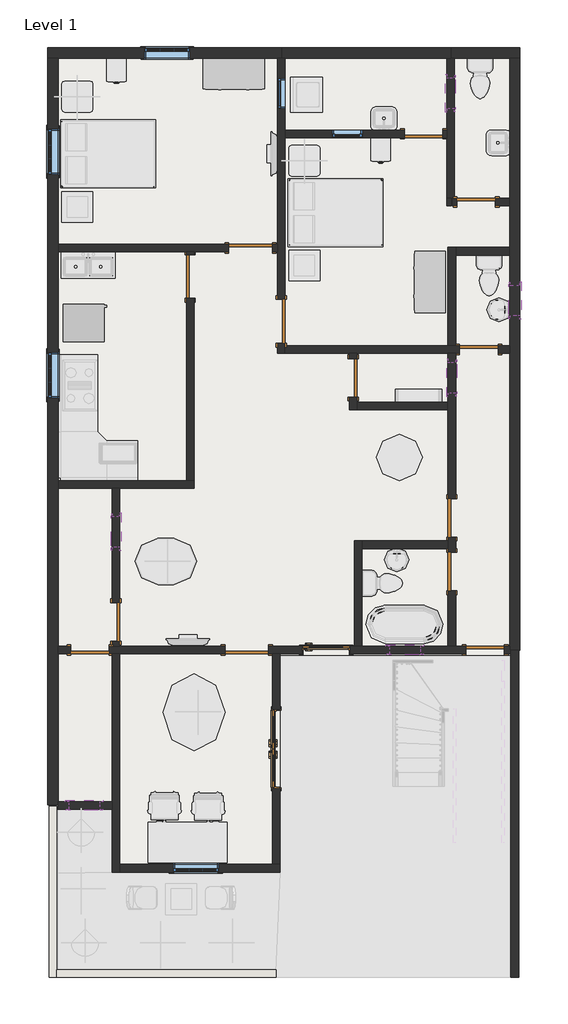
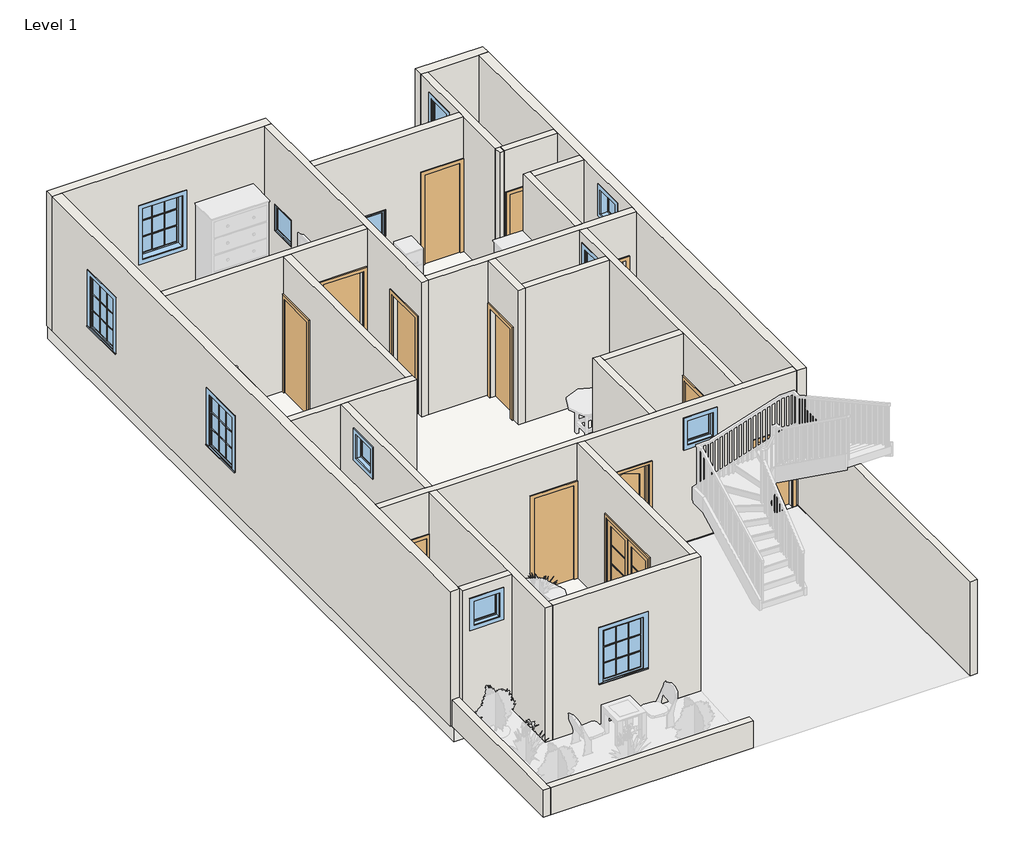
# One storey, part 1 of 3: 30 walls, 15 doors, 12 windows, 1 slab.
"""IFC4 building model written with IfcOpenShell, lengths in millimetres."""

from ifc_helpers import new_model, si_unit, frame, origin, origin_with_axes, place, context, project, spatial, polyline, outline, extrude, faceted_brep, transform, mapped, element, save
from components import door_5d363d20, door_94998e6c, door_1a1933ce, door_255cab33, door_059fdd7e, door_b6e9fca3, door_99d96fc5, window_29c06734, window_5c190c7e, window_aff1bc2a, window_3d781103, window_e41d21a6

model = new_model("IFC4")

# Units and contexts
model_context = context("Model", 3, world=origin())
ifc_project = project(units=[si_unit("LENGTHUNIT", "METRE", prefix="MILLI")], contexts=[model_context])

# Site, building, storey
site = spatial("IfcSite", under=ifc_project)
building = spatial("IfcBuilding", under=site)
storey = spatial("IfcBuildingStorey", under=building, Name="Level 1", Elevation=0.0)

# Doors
placement = place(None, origin())
door_shape = door_5d363d20(model_context)
element("IfcDoor", 1, ObjectType="36\" x 80\"", at=placement, inside=storey, context=model_context, shape_type="MappedRepresentation", body=[
    mapped(door_shape, transform((-9169.2021832, 1057.9854001, 0.0), x_axis=(-1.0, 0.0, 0.0), y_axis=(0.0, -1.0, 0.0), z_axis=(0.0, 0.0, 1.0))),
])
door_2_shape = door_94998e6c(model_context)
element("IfcDoor", 2, ObjectType="Door-Exterior-Double-Full Glass-Wood_Clad : 60\" x 80\"", at=placement, inside=storey, context=model_context, shape_type="MappedRepresentation", body=[
    mapped(door_2_shape, transform((-10162.9771832, -900.9895999, 0.0), x_axis=(0.0, 1.0, 0.0), y_axis=(-1.0, 0.0, 0.0), z_axis=(0.0, 0.0, 1.0))),
])
door_3_shape = door_1a1933ce(model_context)
element("IfcDoor", 3, ObjectType="Single-Flush : 30\" x 68\"", at=placement, inside=storey, context=model_context, shape_type="MappedRepresentation", body=[
    mapped(door_3_shape, transform((-6019.6021832, 1054.8104001, 0.0), x_axis=(1.0, 0.0, 0.0), y_axis=(0.0, 1.0, 0.0), z_axis=(0.0, 0.0, 1.0))),
])
door_4_shape = door_255cab33(model_context)
element("IfcDoor", 4, ObjectType="Single-Flush : 30\" x 80\"", at=placement, inside=storey, context=model_context, shape_type="MappedRepresentation", body=[
    mapped(door_4_shape, transform((-8635.8021832, 6439.6104001, 0.0), x_axis=(0.0, 1.0, 0.0), y_axis=(-1.0, 0.0, 0.0), z_axis=(0.0, 0.0, 1.0))),
])
element("IfcDoor", 5, ObjectType="Single-Flush : 30\" x 80\"", at=placement, inside=storey, context=model_context, shape_type="MappedRepresentation", body=[
    mapped(door_4_shape, transform((-7238.8021832, 11265.6104001, 0.0), x_axis=(1.0, 0.0, 0.0), y_axis=(0.0, 1.0, 0.0), z_axis=(0.0, 0.0, 1.0))),
])
element("IfcDoor", 6, ObjectType="Single-Flush : 30\" x 80\"", at=placement, inside=storey, context=model_context, shape_type="MappedRepresentation", body=[
    mapped(door_4_shape, transform((-6197.4021832, 9919.4104001, 0.0), x_axis=(-1.0, 0.0, 0.0), y_axis=(0.0, -1.0, 0.0), z_axis=(0.0, 0.0, 1.0))),
])
element("IfcDoor", 7, ObjectType="Single-Flush : 30\" x 80\"", at=placement, inside=storey, context=model_context, shape_type="MappedRepresentation", body=[
    mapped(door_4_shape, transform((-6146.6021832, 6998.4104001, 0.0), x_axis=(-1.0, 0.0, 0.0), y_axis=(0.0, -1.0, 0.0), z_axis=(0.0, 0.0, 1.0))),
])
element("IfcDoor", 8, ObjectType="Single-Flush : 30\" x 80\"", at=placement, inside=storey, context=model_context, shape_type="MappedRepresentation", body=[
    mapped(door_4_shape, transform((-6680.0021832, 3671.0104001, 0.0), x_axis=(0.0, -1.0, 0.0), y_axis=(1.0, 0.0, 0.0), z_axis=(0.0, 0.0, 1.0))),
])
element("IfcDoor", 9, ObjectType="Single-Flush : 30\" x 80\"", at=placement, inside=storey, context=model_context, shape_type="MappedRepresentation", body=[
    mapped(door_4_shape, transform((-13842.8021832, 1054.8104001, 0.0), x_axis=(1.0, 0.0, 0.0), y_axis=(0.0, 1.0, 0.0), z_axis=(0.0, 0.0, 1.0))),
])
door_5_shape = door_059fdd7e(model_context)
element("IfcDoor", 10, ObjectType="Single-Flush : 30\" x 80\"", at=placement, inside=storey, context=model_context, shape_type="MappedRepresentation", body=[
    mapped(door_5_shape, transform((-6680.0021832, 2604.2104001, 0.0), x_axis=(0.0, 1.0, 0.0), y_axis=(-1.0, 0.0, 0.0), z_axis=(0.0, 0.0, 1.0))),
])
element("IfcDoor", 11, ObjectType="Single-Flush : 30\" x 80\"", at=placement, inside=storey, context=model_context, shape_type="MappedRepresentation", body=[
    mapped(door_5_shape, transform((-13334.8021832, 1613.6104001, 0.0), x_axis=(0.0, -1.0, 0.0), y_axis=(1.0, 0.0, 0.0), z_axis=(0.0, 0.0, 1.0))),
])
door_6_shape = door_b6e9fca3(model_context)
element("IfcDoor", 12, ObjectType="Single-Flush : 34\" x 84\"", at=placement, inside=storey, context=model_context, shape_type="MappedRepresentation", body=[
    mapped(door_6_shape, transform((-10667.8021832, 9005.0104001, 0.0), x_axis=(1.0, 0.0, 0.0), y_axis=(0.0, 1.0, 0.0), z_axis=(0.0, 0.0, 1.0))),
])
element("IfcDoor", 13, ObjectType="Single-Flush : 34\" x 84\"", at=placement, inside=storey, context=model_context, shape_type="MappedRepresentation", body=[
    mapped(door_6_shape, transform((-11861.6021832, 8446.2104001, 0.0), x_axis=(0.0, 1.0, 0.0), y_axis=(-1.0, 0.0, 0.0), z_axis=(0.0, 0.0, 1.0))),
])
element("IfcDoor", 14, ObjectType="Single-Flush : 34\" x 84\"", at=placement, inside=storey, context=model_context, shape_type="MappedRepresentation", body=[
    mapped(door_6_shape, transform((-10058.2021832, 7557.2104001, 0.0), x_axis=(0.0, -1.0, 0.0), y_axis=(1.0, 0.0, 0.0), z_axis=(0.0, 0.0, 1.0))),
])
door_7_shape = door_99d96fc5(model_context)
element("IfcDoor", 15, ObjectType="Single-Flush : 34\" x 84\"", at=placement, inside=storey, context=model_context, shape_type="MappedRepresentation", body=[
    mapped(door_7_shape, transform((-10744.0021832, 1054.8104001, 0.0), x_axis=(1.0, 0.0, 0.0), y_axis=(0.0, 1.0, 0.0), z_axis=(0.0, 0.0, 1.0))),
])

# Slab
element("IfcSlab", 16, ObjectType="Generic - 12\"", at=placement, inside=storey, context=model_context, shape_type="SweptSolid", body=[
    extrude(outline(polyline([(-5359.2021832, 12967.4104001), (-5359.2021832, 953.2104001), (-10083.6021832, 953.2104001), (-10083.6021832, -3339.3895999), (-13411.0021832, -3339.3895999), (-13411.0021832, -2094.7895999), (-14655.6021832, -2094.7895999), (-14655.6021832, 12967.4104001), (-5359.2021832, 12967.4104001)])), frame((0.0, 0.0, -304.8), z_axis=(0.0, 0.0, 1.0), x_axis=(1.0, 0.0, 0.0)), (0.0, 0.0, 1.0), 304.8),
])

# Walls
element("IfcWall", 17, at=placement, inside=storey, context=model_context, shape_type="Brep", body=[
    faceted_brep([(-14503.2021832, -5422.1895999, 0.0), (-14503.2021832, -5269.7895999, 0.0), (-14503.2021832, -2031.2895999, 0.0), (-14503.2021832, -2031.2895999, 609.6), (-14503.2021832, -5269.7895999, 609.6), (-14503.2021832, -5422.1895999, 609.6), (-14655.6021832, -5422.1895999, 0.0), (-14655.6021832, -5422.1895999, 609.6), (-14655.6021832, -2031.2895999, 609.6), (-14655.6021832, -2031.2895999, 0.0)], [[[0, 1, 2, 3, 4, 5]], [[6, 7, 8, 9]], [[2, 1, 0, 6, 9]], [[3, 2, 9, 8]], [[5, 4, 3, 8, 7]], [[0, 5, 7, 6]]]),
])
element("IfcWall", 18, at=placement, inside=storey, context=model_context, shape_type="SweptSolid", body=[
    extrude(outline(polyline([(-10159.8021832, -5422.1895999), (-14503.2021832, -5422.1895999), (-14503.2021832, -5269.7895999), (-10159.8021832, -5269.7895999), (-10159.8021832, -5422.1895999)])), origin_with_axes(), (0.0, 0.0, 1.0), 609.6),
])
element("IfcWall", 19, at=placement, inside=storey, context=model_context, shape_type="Brep", body=[
    faceted_brep([(-5511.6021832, 1054.8104001, 0.0), (-5511.6021832, 978.6104001, 0.0), (-5511.6021832, -5422.1895999, 0.0), (-5511.6021832, -5422.1895999, 2133.6), (-5511.6021832, 978.6104001, 2133.6), (-5511.6021832, 1054.8104001, 2133.6), (-5359.2021832, 1054.8104001, 0.0), (-5359.2021832, 1054.8104001, 2133.6), (-5359.2021832, -5422.1895999, 2133.6), (-5359.2021832, -5422.1895999, 0.0)], [[[0, 1, 2, 3, 4, 5]], [[6, 7, 8, 9]], [[2, 1, 0, 6, 9]], [[3, 2, 9, 8]], [[5, 4, 3, 8, 7]], [[0, 5, 7, 6]]]),
])
element("IfcWall", 20, ObjectType="Generic - 8\"", at=placement, inside=storey, context=model_context, shape_type="Brep", body=[
    faceted_brep([(-14681.0021832, 12764.2104001, 0.0), (-14477.8021832, 12764.2104001, 0.0), (-10134.4021832, 12764.2104001, 0.0), (-10058.2021832, 12764.2104001, 0.0), (-10058.2021832, 12764.2104001, 1524.0), (-9982.0021832, 12764.2104001, 1524.0), (-9982.0021832, 12764.2104001, 3048.0), (-10134.4021832, 12764.2104001, 3048.0), (-14477.8021832, 12764.2104001, 3048.0), (-14681.0021832, 12764.2104001, 3048.0), (-11861.6021832, 12764.2104001, 2133.6), (-11861.6021832, 12764.2104001, 914.4), (-12776.0021832, 12764.2104001, 914.4), (-12776.0021832, 12764.2104001, 2133.6), (-14681.0021832, 12967.4104001, 0.0), (-14681.0021832, 12967.4104001, 3048.0), (-9982.0021832, 12967.4104001, 3048.0), (-9982.0021832, 12967.4104001, 1524.0), (-10058.2021832, 12967.4104001, 1524.0), (-10058.2021832, 12967.4104001, 0.0), (-11861.6021832, 12967.4104001, 2133.6), (-12776.0021832, 12967.4104001, 2133.6), (-12776.0021832, 12967.4104001, 914.4), (-11861.6021832, 12967.4104001, 914.4)], [[[0, 1, 2, 3, 4, 5, 6, 7, 8, 9], [10, 11, 12, 13]], [[14, 15, 16, 17, 18, 19], [20, 21, 22, 23]], [[3, 2, 1, 0, 14, 19]], [[0, 9, 15, 14]], [[11, 10, 20, 23]], [[12, 11, 23, 22]], [[13, 12, 22, 21]], [[10, 13, 21, 20]], [[4, 3, 19, 18]], [[17, 5, 4, 18]], [[6, 5, 17, 16]], [[9, 8, 7, 6, 16, 15]]]),
])
element("IfcWall", 21, ObjectType="Generic - 8\"", at=placement, inside=storey, context=model_context, shape_type="Brep", body=[
    faceted_brep([(-5537.0021832, 12764.2104001, 0.0), (-5537.0021832, 9995.6104001, 0.0), (-5537.0021832, 9843.2104001, 0.0), (-5537.0021832, 9017.7104001, 0.0), (-5537.0021832, 8865.3104001, 0.0), (-5537.0021832, 7074.6104001, 0.0), (-5537.0021832, 6922.2104001, 0.0), (-5537.0021832, 1131.0104001, 0.0), (-5537.0021832, 1054.8104001, 0.0), (-5537.0021832, 1054.8104001, 2133.6), (-5537.0021832, 978.6104001, 2133.6), (-5537.0021832, 978.6104001, 3048.0), (-5537.0021832, 1131.0104001, 3048.0), (-5537.0021832, 6922.2104001, 3048.0), (-5537.0021832, 7074.6104001, 3048.0), (-5537.0021832, 8865.3104001, 3048.0), (-5537.0021832, 9017.7104001, 3048.0), (-5537.0021832, 9843.2104001, 3048.0), (-5537.0021832, 9995.6104001, 3048.0), (-5537.0021832, 12764.2104001, 3048.0), (-5537.0021832, 7665.1604001, 2768.6), (-5537.0021832, 7665.1604001, 2159.0), (-5537.0021832, 8274.7604001, 2159.0), (-5537.0021832, 8274.7604001, 2768.6), (-5333.8021832, 12764.2104001, 0.0), (-5333.8021832, 12764.2104001, 3048.0), (-5333.8021832, 978.6104001, 3048.0), (-5333.8021832, 978.6104001, 2133.6), (-5333.8021832, 1054.8104001, 2133.6), (-5333.8021832, 1054.8104001, 0.0), (-5333.8021832, 7665.1604001, 2768.6), (-5333.8021832, 8274.7604001, 2768.6), (-5333.8021832, 8274.7604001, 2159.0), (-5333.8021832, 7665.1604001, 2159.0), (-5359.2021832, 1054.8104001, 0.0), (-5511.6021832, 1054.8104001, 0.0), (-5359.2021832, 1054.8104001, 2133.6), (-5511.6021832, 1054.8104001, 2133.6), (-5511.6021832, 978.6104001, 2133.6)], [[[0, 1, 2, 3, 4, 5, 6, 7, 8, 9, 10, 11, 12, 13, 14, 15, 16, 17, 18, 19], [20, 21, 22, 23]], [[24, 25, 26, 27, 28, 29], [30, 31, 32, 33]], [[8, 7, 6, 5, 4, 3, 2, 1, 0, 24, 29, 34, 35]], [[0, 19, 25, 24]], [[21, 20, 30, 33]], [[22, 21, 33, 32]], [[23, 22, 32, 31]], [[20, 23, 31, 30]], [[9, 8, 35, 34, 29, 28, 36, 37]], [[27, 38, 10, 9, 37, 36, 28]], [[11, 10, 38, 27, 26]], [[19, 18, 17, 16, 15, 14, 13, 12, 11, 26, 25]]]),
])
element("IfcWall", 22, ObjectType="Generic - 8\"", at=placement, inside=storey, context=model_context, shape_type="Brep", body=[
    faceted_brep([(-10058.2021832, 12764.2104001, 0.0), (-9982.0021832, 12764.2104001, 0.0), (-6781.6021832, 12764.2104001, 0.0), (-6705.4021832, 12764.2104001, 0.0), (-6705.4021832, 12764.2104001, 1524.0), (-6781.6021832, 12764.2104001, 1524.0), (-9982.0021832, 12764.2104001, 1524.0), (-10058.2021832, 12764.2104001, 1524.0), (-10058.2021832, 12967.4104001, 0.0), (-10058.2021832, 12967.4104001, 1524.0), (-9982.0021832, 12967.4104001, 1524.0), (-6781.6021832, 12967.4104001, 1524.0), (-6705.4021832, 12967.4104001, 1524.0), (-6705.4021832, 12967.4104001, 0.0)], [[[0, 1, 2, 3, 4, 5, 6, 7]], [[8, 9, 10, 11, 12, 13]], [[3, 2, 1, 0, 8, 13]], [[4, 3, 13, 12]], [[7, 6, 5, 4, 12, 11, 10, 9]], [[0, 7, 9, 8]]]),
])
element("IfcWall", 23, ObjectType="Generic - 8\"", at=placement, inside=storey, context=model_context, shape_type="Brep", body=[
    faceted_brep([(-6705.4021832, 12764.2104001, 0.0), (-6629.2021832, 12764.2104001, 0.0), (-5537.0021832, 12764.2104001, 0.0), (-5333.8021832, 12764.2104001, 0.0), (-5333.8021832, 12764.2104001, 3048.0), (-5537.0021832, 12764.2104001, 3048.0), (-6629.2021832, 12764.2104001, 3048.0), (-6781.6021832, 12764.2104001, 3048.0), (-6781.6021832, 12764.2104001, 1524.0), (-6705.4021832, 12764.2104001, 1524.0), (-6705.4021832, 12967.4104001, 0.0), (-6705.4021832, 12967.4104001, 1524.0), (-6781.6021832, 12967.4104001, 1524.0), (-6781.6021832, 12967.4104001, 3048.0), (-5333.8021832, 12967.4104001, 3048.0), (-5333.8021832, 12967.4104001, 0.0)], [[[0, 1, 2, 3, 4, 5, 6, 7, 8, 9]], [[10, 11, 12, 13, 14, 15]], [[3, 2, 1, 0, 10, 15]], [[4, 3, 15, 14]], [[0, 9, 11, 10]], [[8, 12, 11, 9]], [[8, 7, 13, 12]], [[7, 6, 5, 4, 14, 13]]]),
])
element("IfcWall", 24, ObjectType="Generic - 8\"", at=placement, inside=storey, context=model_context, shape_type="Brep", body=[
    faceted_brep([(-14477.8021832, -2005.8895999, 0.0), (-14477.8021832, -1942.3895999, 0.0), (-14477.8021832, 978.6104001, 0.0), (-14477.8021832, 1131.0104001, 0.0), (-14477.8021832, 4255.2104001, 0.0), (-14477.8021832, 4407.6104001, 0.0), (-14477.8021832, 8928.8104001, 0.0), (-14477.8021832, 9081.2104001, 0.0), (-14477.8021832, 12764.2104001, 0.0), (-14477.8021832, 12764.2104001, 3048.0), (-14477.8021832, 9081.2104001, 3048.0), (-14477.8021832, 8928.8104001, 3048.0), (-14477.8021832, 4407.6104001, 3048.0), (-14477.8021832, 4255.2104001, 3048.0), (-14477.8021832, 1131.0104001, 3048.0), (-14477.8021832, 978.6104001, 3048.0), (-14477.8021832, -1942.3895999, 3048.0), (-14477.8021832, -2005.8895999, 3048.0), (-14477.8021832, 11367.2104001, 2133.6), (-14477.8021832, 11367.2104001, 914.4), (-14477.8021832, 10452.8104001, 914.4), (-14477.8021832, 10452.8104001, 2133.6), (-14477.8021832, 6947.6104001, 2133.6), (-14477.8021832, 6947.6104001, 914.4), (-14477.8021832, 6033.2104001, 914.4), (-14477.8021832, 6033.2104001, 2133.6), (-14681.0021832, -2005.8895999, 0.0), (-14681.0021832, -2005.8895999, 3048.0), (-14681.0021832, 12764.2104001, 3048.0), (-14681.0021832, 12764.2104001, 0.0), (-14681.0021832, 11367.2104001, 2133.6), (-14681.0021832, 10452.8104001, 2133.6), (-14681.0021832, 10452.8104001, 914.4), (-14681.0021832, 11367.2104001, 914.4), (-14681.0021832, 6947.6104001, 2133.6), (-14681.0021832, 6033.2104001, 2133.6), (-14681.0021832, 6033.2104001, 914.4), (-14681.0021832, 6947.6104001, 914.4)], [[[0, 1, 2, 3, 4, 5, 6, 7, 8, 9, 10, 11, 12, 13, 14, 15, 16, 17], [18, 19, 20, 21], [22, 23, 24, 25]], [[26, 27, 28, 29], [30, 31, 32, 33], [34, 35, 36, 37]], [[8, 7, 6, 5, 4, 3, 2, 1, 0, 26, 29]], [[0, 17, 27, 26]], [[9, 8, 29, 28]], [[18, 21, 31, 30]], [[21, 20, 32, 31]], [[20, 19, 33, 32]], [[19, 18, 30, 33]], [[22, 25, 35, 34]], [[25, 24, 36, 35]], [[24, 23, 37, 36]], [[23, 22, 34, 37]], [[17, 16, 15, 14, 13, 12, 11, 10, 9, 28, 27]]]),
])
element("IfcWall", 25, ObjectType="INNER 6\"", at=placement, inside=storey, context=model_context, shape_type="Brep", body=[
    faceted_brep([(-10134.4021832, 7125.4104001, 2133.6), (-10134.4021832, 7125.4104001, 0.0), (-10134.4021832, 6922.2104001, 0.0), (-10134.4021832, 6922.2104001, 3048.0), (-10134.4021832, 8928.8104001, 3048.0), (-10134.4021832, 9081.2104001, 3048.0), (-10134.4021832, 12764.2104001, 3048.0), (-10134.4021832, 12764.2104001, 0.0), (-10134.4021832, 9081.2104001, 0.0), (-10134.4021832, 8928.8104001, 0.0), (-10134.4021832, 7989.0104001, 0.0), (-10134.4021832, 7989.0104001, 2133.6), (-10134.4021832, 12370.5104001, 1524.0), (-10134.4021832, 11760.9104001, 1524.0), (-10134.4021832, 11760.9104001, 914.4), (-10134.4021832, 12370.5104001, 914.4), (-9982.0021832, 6922.2104001, 0.0), (-9982.0021832, 7074.6104001, 0.0), (-9982.0021832, 7125.4104001, 0.0), (-9982.0021832, 7125.4104001, 2133.6), (-9982.0021832, 7989.0104001, 2133.6), (-9982.0021832, 7989.0104001, 0.0), (-9982.0021832, 11189.4104001, 0.0), (-9982.0021832, 11341.8104001, 0.0), (-9982.0021832, 12764.2104001, 0.0), (-9982.0021832, 12764.2104001, 1524.0), (-9982.0021832, 12764.2104001, 3048.0), (-9982.0021832, 11341.8104001, 3048.0), (-9982.0021832, 11189.4104001, 3048.0), (-9982.0021832, 7074.6104001, 3048.0), (-9982.0021832, 6922.2104001, 3048.0), (-9982.0021832, 12370.5104001, 1524.0), (-9982.0021832, 12370.5104001, 914.4), (-9982.0021832, 11760.9104001, 914.4), (-9982.0021832, 11760.9104001, 1524.0), (-10058.2021832, 12764.2104001, 0.0)], [[[0, 1, 2, 3, 4, 5, 6, 7, 8, 9, 10, 11], [12, 13, 14, 15]], [[16, 17, 18, 19, 20, 21, 22, 23, 24, 25, 26, 27, 28, 29, 30], [31, 32, 33, 34]], [[2, 1, 18, 17, 16]], [[10, 9, 8, 7, 35, 24, 23, 22, 21]], [[3, 2, 16, 30]], [[19, 18, 1, 0]], [[20, 19, 0, 11]], [[21, 20, 11, 10]], [[32, 31, 12, 15]], [[33, 32, 15, 14]], [[34, 33, 14, 13]], [[31, 34, 13, 12]], [[6, 26, 25, 24, 35, 7]], [[6, 5, 4, 3, 30, 29, 28, 27, 26]]]),
])
element("IfcWall", 26, ObjectType="INNER 6\"", at=placement, inside=storey, context=model_context, shape_type="Brep", body=[
    faceted_brep([(-10134.4021832, 9081.2104001, 0.0), (-10236.0021832, 9081.2104001, 0.0), (-10236.0021832, 9081.2104001, 2133.6), (-11099.6021832, 9081.2104001, 2133.6), (-11099.6021832, 9081.2104001, 0.0), (-14477.8021832, 9081.2104001, 0.0), (-14477.8021832, 9081.2104001, 3048.0), (-10134.4021832, 9081.2104001, 3048.0), (-10236.0021832, 8928.8104001, 2133.6), (-10236.0021832, 8928.8104001, 0.0), (-10134.4021832, 8928.8104001, 0.0), (-10134.4021832, 8928.8104001, 3048.0), (-11785.4021832, 8928.8104001, 3048.0), (-11937.8021832, 8928.8104001, 3048.0), (-14477.8021832, 8928.8104001, 3048.0), (-14477.8021832, 8928.8104001, 0.0), (-11937.8021832, 8928.8104001, 0.0), (-11785.4021832, 8928.8104001, 0.0), (-11099.6021832, 8928.8104001, 0.0), (-11099.6021832, 8928.8104001, 2133.6)], [[[0, 1, 2, 3, 4, 5, 6, 7]], [[8, 9, 10, 11, 12, 13, 14, 15, 16, 17, 18, 19]], [[10, 9, 1, 0]], [[18, 17, 16, 15, 5, 4]], [[0, 7, 11, 10]], [[6, 5, 15, 14]], [[2, 1, 9, 8]], [[3, 2, 8, 19]], [[4, 3, 19, 18]], [[7, 6, 14, 13, 12, 11]]]),
])
element("IfcWall", 27, ObjectType="INNER 6\"", at=placement, inside=storey, context=model_context, shape_type="SweptSolid", body=[
    extrude(outline(polyline([(2032.0, -6857.8021832), (0.0, -6857.8021832), (0.0, -6781.6021832), (3048.0, -6781.6021832), (3048.0, -9982.0021832), (0.0, -9982.0021832), (0.0, -7619.8021832), (2032.0, -7619.8021832), (2032.0, -6857.8021832)]), holes=[polyline([(1524.0, -9054.9021832), (1524.0, -8445.3021832), (914.4, -8445.3021832), (914.4, -9054.9021832), (1524.0, -9054.9021832)])]), frame((0.0, 11189.4104001, 0.0), z_axis=(0.0, 1.0, 0.0), x_axis=(0.0, 0.0, 1.0)), (0.0, 0.0, 1.0), 152.4),
])
element("IfcWall", 28, ObjectType="INNER 6\"", at=placement, inside=storey, context=model_context, shape_type="Brep", body=[
    faceted_brep([(-6629.2021832, 9995.6104001, 0.0), (-6629.2021832, 12764.2104001, 0.0), (-6629.2021832, 12764.2104001, 3048.0), (-6629.2021832, 9995.6104001, 3048.0), (-6629.2021832, 12370.5104001, 2768.6), (-6629.2021832, 12370.5104001, 2159.0), (-6629.2021832, 11760.9104001, 2159.0), (-6629.2021832, 11760.9104001, 2768.6), (-6781.6021832, 9995.6104001, 0.0), (-6781.6021832, 9995.6104001, 3048.0), (-6781.6021832, 11189.4104001, 3048.0), (-6781.6021832, 11341.8104001, 3048.0), (-6781.6021832, 12764.2104001, 3048.0), (-6781.6021832, 12764.2104001, 1524.0), (-6781.6021832, 12764.2104001, 0.0), (-6781.6021832, 11341.8104001, 0.0), (-6781.6021832, 11189.4104001, 0.0), (-6781.6021832, 12370.5104001, 2768.6), (-6781.6021832, 11760.9104001, 2768.6), (-6781.6021832, 11760.9104001, 2159.0), (-6781.6021832, 12370.5104001, 2159.0), (-6692.7021832, 9995.6104001, 0.0), (-6705.4021832, 12764.2104001, 0.0), (-6692.7021832, 9995.6104001, 3048.0)], [[[0, 1, 2, 3], [4, 5, 6, 7]], [[8, 9, 10, 11, 12, 13, 14, 15, 16], [17, 18, 19, 20]], [[1, 0, 21, 8, 16, 15, 14, 22]], [[0, 3, 23, 9, 8, 21]], [[5, 4, 17, 20]], [[6, 5, 20, 19]], [[7, 6, 19, 18]], [[4, 7, 18, 17]], [[1, 22, 14, 13, 12, 2]], [[3, 2, 12, 11, 10, 9, 23]]]),
])
element("IfcWall", 29, ObjectType="INNER 6\"", at=placement, inside=storey, context=model_context, shape_type="SweptSolid", body=[
    extrude(outline(polyline([(-6692.7021832, 9843.2104001), (-6781.6021832, 9843.2104001), (-6781.6021832, 9995.6104001), (-6692.7021832, 9995.6104001), (-6692.7021832, 9843.2104001)])), origin_with_axes(), (0.0, 0.0, 1.0), 3048.0),
])
element("IfcWall", 30, ObjectType="INNER 6\"", at=placement, inside=storey, context=model_context, shape_type="Brep", body=[
    faceted_brep([(-9982.0021832, 6922.2104001, 0.0), (-8712.0021832, 6922.2104001, 0.0), (-8559.6021832, 6922.2104001, 0.0), (-6756.2021832, 6922.2104001, 0.0), (-6603.8021832, 6922.2104001, 0.0), (-6527.6021832, 6922.2104001, 0.0), (-6527.6021832, 6922.2104001, 2032.0), (-5765.6021832, 6922.2104001, 2032.0), (-5765.6021832, 6922.2104001, 0.0), (-5537.0021832, 6922.2104001, 0.0), (-5537.0021832, 6922.2104001, 3048.0), (-6603.8021832, 6922.2104001, 3048.0), (-6756.2021832, 6922.2104001, 3048.0), (-8559.6021832, 6922.2104001, 3048.0), (-8712.0021832, 6922.2104001, 3048.0), (-9982.0021832, 6922.2104001, 3048.0), (-6527.6021832, 7074.6104001, 2032.0), (-6527.6021832, 7074.6104001, 0.0), (-6603.8021832, 7074.6104001, 0.0), (-6756.2021832, 7074.6104001, 0.0), (-9982.0021832, 7074.6104001, 0.0), (-9982.0021832, 7074.6104001, 3048.0), (-6756.2021832, 7074.6104001, 3048.0), (-6603.8021832, 7074.6104001, 3048.0), (-5537.0021832, 7074.6104001, 3048.0), (-5537.0021832, 7074.6104001, 0.0), (-5765.6021832, 7074.6104001, 0.0), (-5765.6021832, 7074.6104001, 2032.0)], [[[0, 1, 2, 3, 4, 5, 6, 7, 8, 9, 10, 11, 12, 13, 14, 15]], [[16, 17, 18, 19, 20, 21, 22, 23, 24, 25, 26, 27]], [[26, 25, 9, 8]], [[20, 19, 18, 17, 5, 4, 3, 2, 1, 0]], [[0, 15, 21, 20]], [[10, 9, 25, 24]], [[6, 5, 17, 16]], [[7, 6, 16, 27]], [[8, 7, 27, 26]], [[15, 14, 13, 12, 11, 10, 24, 23, 22, 21]]]),
])
element("IfcWall", 31, ObjectType="INNER 6\"", at=placement, inside=storey, context=model_context, shape_type="Brep", body=[
    faceted_brep([(-6603.8021832, 2985.2104001, 2032.0), (-6603.8021832, 2985.2104001, 0.0), (-6603.8021832, 3290.0104001, 0.0), (-6603.8021832, 3290.0104001, 2032.0), (-6603.8021832, 4052.0104001, 2032.0), (-6603.8021832, 4052.0104001, 0.0), (-6603.8021832, 6922.2104001, 0.0), (-6603.8021832, 6922.2104001, 3048.0), (-6603.8021832, 1131.0104001, 3048.0), (-6603.8021832, 1131.0104001, 0.0), (-6603.8021832, 2223.2104001, 0.0), (-6603.8021832, 2223.2104001, 2032.0), (-6603.8021832, 6744.4104001, 2768.6), (-6603.8021832, 6744.4104001, 2159.0), (-6603.8021832, 6134.8104001, 2159.0), (-6603.8021832, 6134.8104001, 2768.6), (-6756.2021832, 3290.0104001, 0.0), (-6756.2021832, 3213.8104001, 0.0), (-6756.2021832, 3061.4104001, 0.0), (-6756.2021832, 2985.2104001, 0.0), (-6756.2021832, 2985.2104001, 2032.0), (-6756.2021832, 2223.2104001, 2032.0), (-6756.2021832, 2223.2104001, 0.0), (-6756.2021832, 1131.0104001, 0.0), (-6756.2021832, 1131.0104001, 3048.0), (-6756.2021832, 3061.4104001, 3048.0), (-6756.2021832, 3213.8104001, 3048.0), (-6756.2021832, 5804.6104001, 3048.0), (-6756.2021832, 5957.0104001, 3048.0), (-6756.2021832, 6922.2104001, 3048.0), (-6756.2021832, 6922.2104001, 0.0), (-6756.2021832, 5957.0104001, 0.0), (-6756.2021832, 5804.6104001, 0.0), (-6756.2021832, 4052.0104001, 0.0), (-6756.2021832, 4052.0104001, 2032.0), (-6756.2021832, 3290.0104001, 2032.0), (-6756.2021832, 6744.4104001, 2768.6), (-6756.2021832, 6134.8104001, 2768.6), (-6756.2021832, 6134.8104001, 2159.0), (-6756.2021832, 6744.4104001, 2159.0)], [[[0, 1, 2, 3, 4, 5, 6, 7, 8, 9, 10, 11], [12, 13, 14, 15]], [[16, 17, 18, 19, 20, 21, 22, 23, 24, 25, 26, 27, 28, 29, 30, 31, 32, 33, 34, 35], [36, 37, 38, 39]], [[33, 32, 31, 30, 6, 5]], [[10, 9, 23, 22]], [[2, 1, 19, 18, 17, 16]], [[9, 8, 24, 23]], [[7, 6, 30, 29]], [[3, 2, 16, 35]], [[4, 3, 35, 34]], [[5, 4, 34, 33]], [[20, 19, 1, 0]], [[21, 20, 0, 11]], [[22, 21, 11, 10]], [[13, 12, 36, 39]], [[14, 13, 39, 38]], [[15, 14, 38, 37]], [[12, 15, 37, 36]], [[8, 7, 29, 28, 27, 26, 25, 24]]]),
])
element("IfcWall", 32, ObjectType="INNER 6\"", at=placement, inside=storey, context=model_context, shape_type="Brep", body=[
    faceted_brep([(-14477.8021832, 1131.0104001, 0.0), (-14477.8021832, 1131.0104001, 3048.0), (-13411.0021832, 1131.0104001, 3048.0), (-13258.6021832, 1131.0104001, 3048.0), (-8610.4021832, 1131.0104001, 3048.0), (-8458.0021832, 1131.0104001, 3048.0), (-6756.2021832, 1131.0104001, 3048.0), (-6603.8021832, 1131.0104001, 3048.0), (-5537.0021832, 1131.0104001, 3048.0), (-5537.0021832, 1131.0104001, 2133.6), (-5537.0021832, 1131.0104001, 0.0), (-5638.6021832, 1131.0104001, 0.0), (-5638.6021832, 1131.0104001, 1727.2), (-6400.6021832, 1131.0104001, 1727.2), (-6400.6021832, 1131.0104001, 0.0), (-6603.8021832, 1131.0104001, 0.0), (-6756.2021832, 1131.0104001, 0.0), (-8458.0021832, 1131.0104001, 0.0), (-8610.4021832, 1131.0104001, 0.0), (-8686.6021832, 1131.0104001, 0.0), (-8686.6021832, 1131.0104001, 2057.4), (-9651.8021832, 1131.0104001, 2057.4), (-9651.8021832, 1131.0104001, 0.0), (-10312.2021832, 1131.0104001, 0.0), (-10312.2021832, 1131.0104001, 2133.6), (-11175.8021832, 1131.0104001, 2133.6), (-11175.8021832, 1131.0104001, 0.0), (-13258.6021832, 1131.0104001, 0.0), (-13411.0021832, 1131.0104001, 0.0), (-13461.8021832, 1131.0104001, 0.0), (-13461.8021832, 1131.0104001, 2032.0), (-14223.8021832, 1131.0104001, 2032.0), (-14223.8021832, 1131.0104001, 0.0), (-7302.3021832, 1131.0104001, 2768.6), (-7911.9021832, 1131.0104001, 2768.6), (-7911.9021832, 1131.0104001, 2159.0), (-7302.3021832, 1131.0104001, 2159.0), (-14477.8021832, 978.6104001, 3048.0), (-14477.8021832, 978.6104001, 0.0), (-14223.8021832, 978.6104001, 0.0), (-14223.8021832, 978.6104001, 2032.0), (-13461.8021832, 978.6104001, 2032.0), (-13461.8021832, 978.6104001, 0.0), (-13411.0021832, 978.6104001, 0.0), (-13258.6021832, 978.6104001, 0.0), (-11175.8021832, 978.6104001, 0.0), (-11175.8021832, 978.6104001, 2133.6), (-10312.2021832, 978.6104001, 2133.6), (-10312.2021832, 978.6104001, 0.0), (-10236.0021832, 978.6104001, 0.0), (-10083.6021832, 978.6104001, 0.0), (-9651.8021832, 978.6104001, 0.0), (-9651.8021832, 978.6104001, 2057.4), (-8686.6021832, 978.6104001, 2057.4), (-8686.6021832, 978.6104001, 0.0), (-6400.6021832, 978.6104001, 0.0), (-6400.6021832, 978.6104001, 1727.2), (-5638.6021832, 978.6104001, 1727.2), (-5638.6021832, 978.6104001, 0.0), (-5511.6021832, 978.6104001, 0.0), (-5511.6021832, 978.6104001, 2133.6), (-5537.0021832, 978.6104001, 2133.6), (-5537.0021832, 978.6104001, 3048.0), (-10083.6021832, 978.6104001, 3048.0), (-10236.0021832, 978.6104001, 3048.0), (-13258.6021832, 978.6104001, 3048.0), (-13411.0021832, 978.6104001, 3048.0), (-7302.3021832, 978.6104001, 2768.6), (-7302.3021832, 978.6104001, 2159.0), (-7911.9021832, 978.6104001, 2159.0), (-7911.9021832, 978.6104001, 2768.6), (-5537.0021832, 1054.8104001, 0.0), (-5511.6021832, 1054.8104001, 0.0), (-5511.6021832, 1054.8104001, 2133.6), (-5537.0021832, 1054.8104001, 2133.6)], [[[0, 1, 2, 3, 4, 5, 6, 7, 8, 9, 10, 11, 12, 13, 14, 15, 16, 17, 18, 19, 20, 21, 22, 23, 24, 25, 26, 27, 28, 29, 30, 31, 32], [33, 34, 35, 36]], [[37, 38, 39, 40, 41, 42, 43, 44, 45, 46, 47, 48, 49, 50, 51, 52, 53, 54, 55, 56, 57, 58, 59, 60, 61, 62, 63, 64, 65, 66], [67, 68, 69, 70]], [[38, 0, 32, 39]], [[58, 11, 10, 71, 72, 59]], [[14, 55, 54, 19, 18, 17, 16, 15]], [[42, 29, 28, 27, 26, 45, 44, 43]], [[48, 23, 22, 51, 50, 49]], [[1, 0, 38, 37]], [[12, 11, 58, 57]], [[13, 12, 57, 56]], [[14, 13, 56, 55]], [[30, 29, 42, 41]], [[31, 30, 41, 40]], [[32, 31, 40, 39]], [[24, 23, 48, 47]], [[25, 24, 47, 46]], [[26, 25, 46, 45]], [[21, 52, 51, 22]], [[52, 21, 20, 53]], [[53, 20, 19, 54]], [[68, 67, 33, 36]], [[69, 68, 36, 35]], [[70, 69, 35, 34]], [[67, 70, 34, 33]], [[61, 60, 73, 74]], [[10, 9, 74, 71]], [[9, 8, 62, 61, 74]], [[8, 7, 6, 5, 4, 3, 2, 1, 37, 66, 65, 64, 63, 62]], [[74, 73, 72, 71]], [[60, 59, 72, 73]]]),
])
element("IfcWall", 33, ObjectType="INNER 6\"", at=placement, inside=storey, context=model_context, shape_type="Brep", body=[
    faceted_brep([(-13411.0021832, 978.6104001, 0.0), (-13411.0021832, -1942.3895999, 0.0), (-13411.0021832, -2094.7895999, 0.0), (-13411.0021832, -3339.3895999, 0.0), (-13411.0021832, -3339.3895999, 3048.0), (-13411.0021832, -2094.7895999, 3048.0), (-13411.0021832, -1942.3895999, 3048.0), (-13411.0021832, 978.6104001, 3048.0), (-13258.6021832, 978.6104001, 0.0), (-13258.6021832, 978.6104001, 3048.0), (-13258.6021832, -3186.9895999, 3048.0), (-13258.6021832, -3339.3895999, 3048.0), (-13258.6021832, -3339.3895999, 0.0), (-13258.6021832, -3186.9895999, 0.0)], [[[0, 1, 2, 3, 4, 5, 6, 7]], [[8, 9, 10, 11, 12, 13]], [[3, 2, 1, 0, 8, 13, 12]], [[0, 7, 9, 8]], [[4, 3, 12, 11]], [[7, 6, 5, 4, 11, 10, 9]]]),
])
element("IfcWall", 34, ObjectType="INNER 6\"", at=placement, inside=storey, context=model_context, shape_type="Brep", body=[
    faceted_brep([(-13411.0021832, -1942.3895999, 0.0), (-14477.8021832, -1942.3895999, 0.0), (-14477.8021832, -1942.3895999, 3048.0), (-13411.0021832, -1942.3895999, 3048.0), (-13652.3021832, -1942.3895999, 2768.6), (-14261.9021832, -1942.3895999, 2768.6), (-14261.9021832, -1942.3895999, 2159.0), (-13652.3021832, -1942.3895999, 2159.0), (-13411.0021832, -2094.7895999, 0.0), (-13411.0021832, -2094.7895999, 3048.0), (-14477.8021832, -2094.7895999, 3048.0), (-14477.8021832, -2094.7895999, 0.0), (-13652.3021832, -2094.7895999, 2768.6), (-13652.3021832, -2094.7895999, 2159.0), (-14261.9021832, -2094.7895999, 2159.0), (-14261.9021832, -2094.7895999, 2768.6), (-14477.8021832, -2005.8895999, 0.0), (-14477.8021832, -2005.8895999, 3048.0)], [[[0, 1, 2, 3], [4, 5, 6, 7]], [[8, 9, 10, 11], [12, 13, 14, 15]], [[1, 0, 8, 11, 16]], [[0, 3, 9, 8]], [[2, 1, 16, 11, 10, 17]], [[13, 12, 4, 7]], [[14, 13, 7, 6]], [[15, 14, 6, 5]], [[12, 15, 5, 4]], [[3, 2, 17, 10, 9]]]),
])
element("IfcWall", 35, ObjectType="INNER 6\"", at=placement, inside=storey, context=model_context, shape_type="Brep", body=[
    faceted_brep([(-13258.6021832, -3339.3895999, 0.0), (-10083.6021832, -3339.3895999, 0.0), (-10083.6021832, -3339.3895999, 3048.0), (-13258.6021832, -3339.3895999, 3048.0), (-12204.5021832, -3339.3895999, 2133.6), (-11290.1021832, -3339.3895999, 2133.6), (-11290.1021832, -3339.3895999, 914.4), (-12204.5021832, -3339.3895999, 914.4), (-13258.6021832, -3186.9895999, 0.0), (-13258.6021832, -3186.9895999, 3048.0), (-10236.0021832, -3186.9895999, 3048.0), (-10083.6021832, -3186.9895999, 3048.0), (-10083.6021832, -3186.9895999, 0.0), (-10236.0021832, -3186.9895999, 0.0), (-12204.5021832, -3186.9895999, 2133.6), (-12204.5021832, -3186.9895999, 914.4), (-11290.1021832, -3186.9895999, 914.4), (-11290.1021832, -3186.9895999, 2133.6)], [[[0, 1, 2, 3], [4, 5, 6, 7]], [[8, 9, 10, 11, 12, 13], [14, 15, 16, 17]], [[1, 0, 8, 13, 12]], [[0, 3, 9, 8]], [[2, 1, 12, 11]], [[15, 14, 4, 7]], [[16, 15, 7, 6]], [[17, 16, 6, 5]], [[14, 17, 5, 4]], [[3, 2, 11, 10, 9]]]),
])
element("IfcWall", 36, ObjectType="INNER 6\"", at=placement, inside=storey, context=model_context, shape_type="Brep", body=[
    faceted_brep([(-10083.6021832, -3186.9895999, 3048.0), (-10083.6021832, -3186.9895999, 0.0), (-10083.6021832, -1688.3895999, 0.0), (-10083.6021832, -1688.3895999, 2057.4), (-10083.6021832, -113.5895999, 2057.4), (-10083.6021832, -113.5895999, 0.0), (-10083.6021832, 978.6104001, 0.0), (-10083.6021832, 978.6104001, 3048.0), (-10083.6021832, 953.2104001, 3048.0), (-10236.0021832, -3186.9895999, 3048.0), (-10236.0021832, 978.6104001, 3048.0), (-10236.0021832, 978.6104001, 0.0), (-10236.0021832, -113.5895999, 0.0), (-10236.0021832, -113.5895999, 2057.4), (-10236.0021832, -1688.3895999, 2057.4), (-10236.0021832, -1688.3895999, 0.0), (-10236.0021832, -3186.9895999, 0.0)], [[[0, 1, 2, 3, 4, 5, 6, 7, 8]], [[9, 10, 11, 12, 13, 14, 15, 16]], [[1, 16, 15, 2]], [[11, 6, 5, 12]], [[1, 0, 9, 16]], [[7, 6, 11, 10]], [[4, 13, 12, 5]], [[13, 4, 3, 14]], [[14, 3, 2, 15]], [[10, 9, 0, 8, 7]]]),
])
element("IfcWall", 37, ObjectType="INNER 6\"", at=placement, inside=storey, context=model_context, shape_type="SweptSolid", body=[
    extrude(outline(polyline([(1232.6104001, 2032.0), (1232.6104001, 0.0), (1131.0104001, 0.0), (1131.0104001, 3048.0), (4255.2104001, 3048.0), (4255.2104001, 0.0), (1994.6104001, 0.0), (1994.6104001, 2032.0), (1232.6104001, 2032.0)]), holes=[polyline([(3086.8104001, 2768.6), (3086.8104001, 2159.0), (3696.4104001, 2159.0), (3696.4104001, 2768.6), (3086.8104001, 2768.6)])]), frame((-13411.0021832, 0.0, 0.0), z_axis=(1.0, 0.0, 0.0), x_axis=(0.0, 1.0, 0.0)), (0.0, 0.0, 1.0), 152.4),
])
element("IfcWall", 38, ObjectType="INNER 6\"", at=placement, inside=storey, context=model_context, shape_type="Brep", body=[
    faceted_brep([(-11785.4021832, 4407.6104001, 0.0), (-11937.8021832, 4407.6104001, 0.0), (-14477.8021832, 4407.6104001, 0.0), (-14477.8021832, 4407.6104001, 3048.0), (-11937.8021832, 4407.6104001, 3048.0), (-11785.4021832, 4407.6104001, 3048.0), (-11785.4021832, 4255.2104001, 0.0), (-11785.4021832, 4255.2104001, 3048.0), (-13258.6021832, 4255.2104001, 3048.0), (-13411.0021832, 4255.2104001, 3048.0), (-14477.8021832, 4255.2104001, 3048.0), (-14477.8021832, 4255.2104001, 0.0), (-13411.0021832, 4255.2104001, 0.0), (-13258.6021832, 4255.2104001, 0.0)], [[[0, 1, 2, 3, 4, 5]], [[6, 7, 8, 9, 10, 11, 12, 13]], [[2, 1, 0, 6, 13, 12, 11]], [[3, 2, 11, 10]], [[0, 5, 7, 6]], [[5, 4, 3, 10, 9, 8, 7]]]),
])
element("IfcWall", 39, ObjectType="INNER 6\"", at=placement, inside=storey, context=model_context, shape_type="SweptSolid", body=[
    extrude(outline(polyline([(8928.8104001, 0.0), (8878.0104001, 0.0), (8878.0104001, 2133.6), (8014.4104001, 2133.6), (8014.4104001, 0.0), (4407.6104001, 0.0), (4407.6104001, 3048.0), (8928.8104001, 3048.0), (8928.8104001, 0.0)])), frame((-11937.8021832, 0.0, 0.0), z_axis=(1.0, 0.0, 0.0), x_axis=(0.0, 1.0, 0.0)), (0.0, 0.0, 1.0), 152.4),
])
element("IfcWall", 40, ObjectType="INNER 6\"", at=placement, inside=storey, context=model_context, shape_type="Brep", body=[
    faceted_brep([(-8458.0021832, 1131.0104001, 0.0), (-8458.0021832, 3061.4104001, 0.0), (-8458.0021832, 3213.8104001, 0.0), (-8458.0021832, 3213.8104001, 3048.0), (-8458.0021832, 3061.4104001, 3048.0), (-8458.0021832, 1131.0104001, 3048.0), (-8610.4021832, 1131.0104001, 0.0), (-8610.4021832, 1131.0104001, 3048.0), (-8610.4021832, 3213.8104001, 3048.0), (-8610.4021832, 3213.8104001, 0.0)], [[[0, 1, 2, 3, 4, 5]], [[6, 7, 8, 9]], [[2, 1, 0, 6, 9]], [[0, 5, 7, 6]], [[3, 2, 9, 8]], [[5, 4, 3, 8, 7]]]),
])
element("IfcWall", 41, ObjectType="INNER 6\"", at=placement, inside=storey, context=model_context, shape_type="SweptSolid", body=[
    extrude(outline(polyline([(-6756.2021832, 3061.4104001), (-8458.0021832, 3061.4104001), (-8458.0021832, 3213.8104001), (-6756.2021832, 3213.8104001), (-6756.2021832, 3061.4104001)])), origin_with_axes(), (0.0, 0.0, 1.0), 3048.0),
])
element("IfcWall", 42, ObjectType="INNER 6\"", at=placement, inside=storey, context=model_context, shape_type="Brep", body=[
    faceted_brep([(-8712.0021832, 6922.2104001, 0.0), (-8712.0021832, 6820.6104001, 0.0), (-8712.0021832, 6820.6104001, 2032.0), (-8712.0021832, 6058.6104001, 2032.0), (-8712.0021832, 6058.6104001, 0.0), (-8712.0021832, 5804.6104001, 0.0), (-8712.0021832, 5804.6104001, 3048.0), (-8712.0021832, 6922.2104001, 3048.0), (-8559.6021832, 6820.6104001, 2032.0), (-8559.6021832, 6820.6104001, 0.0), (-8559.6021832, 6922.2104001, 0.0), (-8559.6021832, 6922.2104001, 3048.0), (-8559.6021832, 5957.0104001, 3048.0), (-8559.6021832, 5804.6104001, 3048.0), (-8559.6021832, 5804.6104001, 0.0), (-8559.6021832, 5957.0104001, 0.0), (-8559.6021832, 6058.6104001, 0.0), (-8559.6021832, 6058.6104001, 2032.0)], [[[0, 1, 2, 3, 4, 5, 6, 7]], [[8, 9, 10, 11, 12, 13, 14, 15, 16, 17]], [[10, 9, 1, 0]], [[16, 15, 14, 5, 4]], [[0, 7, 11, 10]], [[6, 5, 14, 13]], [[2, 1, 9, 8]], [[3, 2, 8, 17]], [[4, 3, 17, 16]], [[7, 6, 13, 12, 11]]]),
])
element("IfcWall", 43, ObjectType="INNER 6\"", at=placement, inside=storey, context=model_context, shape_type="SweptSolid", body=[
    extrude(outline(polyline([(-6756.2021832, 5804.6104001), (-8559.6021832, 5804.6104001), (-8559.6021832, 5957.0104001), (-6756.2021832, 5957.0104001), (-6756.2021832, 5804.6104001)])), origin_with_axes(), (0.0, 0.0, 1.0), 3048.0),
])
element("IfcWall", 44, ObjectType="INNER 6\"", at=placement, inside=storey, context=model_context, shape_type="Brep", body=[
    faceted_brep([(-6603.8021832, 7074.6104001, 0.0), (-6603.8021832, 8865.3104001, 0.0), (-6603.8021832, 9017.7104001, 0.0), (-6603.8021832, 9017.7104001, 3048.0), (-6603.8021832, 8865.3104001, 3048.0), (-6603.8021832, 7074.6104001, 3048.0), (-6756.2021832, 7074.6104001, 0.0), (-6756.2021832, 7074.6104001, 3048.0), (-6756.2021832, 9017.7104001, 3048.0), (-6756.2021832, 9017.7104001, 0.0)], [[[0, 1, 2, 3, 4, 5]], [[6, 7, 8, 9]], [[2, 1, 0, 6, 9]], [[3, 2, 9, 8]], [[0, 5, 7, 6]], [[5, 4, 3, 8, 7]]]),
])
element("IfcWall", 45, ObjectType="INNER 6\"", at=placement, inside=storey, context=model_context, shape_type="SweptSolid", body=[
    extrude(outline(polyline([(0.0, -6667.3021832), (0.0, -6578.4021832), (2032.0, -6578.4021832), (2032.0, -5816.4021832), (0.0, -5816.4021832), (0.0, -5537.0021832), (3048.0, -5537.0021832), (3048.0, -6667.3021832), (0.0, -6667.3021832)])), frame((0.0, 9843.2104001, 0.0), z_axis=(0.0, 1.0, 0.0), x_axis=(0.0, 0.0, 1.0)), (0.0, 0.0, 1.0), 152.4),
])
element("IfcWall", 46, ObjectType="INNER 6\"", at=placement, inside=storey, context=model_context, shape_type="SweptSolid", body=[
    extrude(outline(polyline([(-5537.0021832, 8865.3104001), (-6603.8021832, 8865.3104001), (-6603.8021832, 9017.7104001), (-5537.0021832, 9017.7104001), (-5537.0021832, 8865.3104001)])), origin_with_axes(), (0.0, 0.0, 1.0), 3048.0),
])

# Windows
window_shape = window_29c06734(model_context)
element("IfcWindow", 47, ObjectType="Casement 3x3 with Trim : 36\" x 48\"", at=placement, inside=storey, context=model_context, shape_type="MappedRepresentation", body=[
    mapped(window_shape, transform((-12318.8021832, 12865.8104001, 0.0), x_axis=(1.0, 0.0, 0.0), y_axis=(0.0, 1.0, 0.0), z_axis=(0.0, 0.0, 1.0))),
])
element("IfcWindow", 48, ObjectType="Casement 3x3 with Trim : 36\" x 48\"", at=placement, inside=storey, context=model_context, shape_type="MappedRepresentation", body=[
    mapped(window_shape, transform((-14579.4021832, 10910.0104001, 0.0), x_axis=(0.0, 1.0, 0.0), y_axis=(-1.0, 0.0, 0.0), z_axis=(0.0, 0.0, 1.0))),
])
element("IfcWindow", 49, ObjectType="Casement 3x3 with Trim : 36\" x 48\"", at=placement, inside=storey, context=model_context, shape_type="MappedRepresentation", body=[
    mapped(window_shape, transform((-14579.4021832, 6490.4104001, 0.0), x_axis=(0.0, 1.0, 0.0), y_axis=(-1.0, 0.0, 0.0), z_axis=(0.0, 0.0, 1.0))),
])
window_2_shape = window_5c190c7e(model_context)
element("IfcWindow", 50, ObjectType="Casement 3x3 with Trim : 36\" x 48\"", at=placement, inside=storey, context=model_context, shape_type="MappedRepresentation", body=[
    mapped(window_2_shape, transform((-11747.3021832, -3263.1895999, 0.0), x_axis=(-1.0, 0.0, 0.0), y_axis=(0.0, -1.0, 0.0), z_axis=(0.0, 0.0, 1.0))),
])
window_3_shape = window_aff1bc2a(model_context)
element("IfcWindow", 51, ObjectType="Fixed : 24\" x 24\"", at=placement, inside=storey, context=model_context, shape_type="MappedRepresentation", body=[
    mapped(window_3_shape, transform((-10058.2021832, 12103.8104001, 0.0), x_axis=(0.0, 1.0, 0.0), y_axis=(-1.0, 0.0, 0.0), z_axis=(0.0, 0.0, 1.0))),
])
element("IfcWindow", 52, ObjectType="Fixed : 24\" x 24\"", at=placement, inside=storey, context=model_context, shape_type="MappedRepresentation", body=[
    mapped(window_3_shape, transform((-8788.2021832, 11265.6104001, 0.0), x_axis=(-1.0, 0.0, 0.0), y_axis=(0.0, -1.0, 0.0), z_axis=(0.0, 0.0, 1.0))),
])
window_4_shape = window_3d781103(model_context)
element("IfcWindow", 53, ObjectType="Transom with Trim : 24\" x 24\"", at=placement, inside=storey, context=model_context, shape_type="MappedRepresentation", body=[
    mapped(window_4_shape, transform((-6705.4021832, 12103.8104001, 0.0), x_axis=(0.0, 1.0, 0.0), y_axis=(-1.0, 0.0, 0.0), z_axis=(0.0, 0.0, 1.0))),
])
element("IfcWindow", 54, ObjectType="Transom with Trim : 24\" x 24\"", at=placement, inside=storey, context=model_context, shape_type="MappedRepresentation", body=[
    mapped(window_4_shape, transform((-6680.0021832, 6477.7104001, 0.0), x_axis=(0.0, 1.0, 0.0), y_axis=(-1.0, 0.0, 0.0), z_axis=(0.0, 0.0, 1.0))),
])
element("IfcWindow", 55, ObjectType="Transom with Trim : 24\" x 24\"", at=placement, inside=storey, context=model_context, shape_type="MappedRepresentation", body=[
    mapped(window_4_shape, transform((-7569.0021832, 1054.8104001, 0.0), x_axis=(1.0, 0.0, 0.0), y_axis=(0.0, 1.0, 0.0), z_axis=(0.0, 0.0, 1.0))),
])
element("IfcWindow", 56, ObjectType="Transom with Trim : 24\" x 24\"", at=placement, inside=storey, context=model_context, shape_type="MappedRepresentation", body=[
    mapped(window_4_shape, transform((-13919.0021832, -2018.5895999, 0.0), x_axis=(1.0, 0.0, 0.0), y_axis=(0.0, 1.0, 0.0), z_axis=(0.0, 0.0, 1.0))),
])
element("IfcWindow", 57, ObjectType="Transom with Trim : 24\" x 24\"", at=placement, inside=storey, context=model_context, shape_type="MappedRepresentation", body=[
    mapped(window_4_shape, transform((-13334.8021832, 3353.5104001, 0.0), x_axis=(0.0, -1.0, 0.0), y_axis=(1.0, 0.0, 0.0), z_axis=(0.0, 0.0, 1.0))),
])
window_5_shape = window_e41d21a6(model_context)
element("IfcWindow", 58, ObjectType="Transom with Trim : 24\" x 24\"", at=placement, inside=storey, context=model_context, shape_type="MappedRepresentation", body=[
    mapped(window_5_shape, transform((-5435.4021832, 7931.8604001, 0.0), x_axis=(0.0, -1.0, 0.0), y_axis=(1.0, 0.0, 0.0), z_axis=(0.0, 0.0, 1.0))),
])

save(model, "model.ifc")

# Revit data of these elements
# Type "36\" x 80\""
#   Type Mark = "9"
#   Assembly Code = "B2030100"
#   Analytic Construction = "French door, wood frame with single glass"
#   Threshold Offset [instance default] = 0' - 0 1/2"
#   Thickness = 0' - 1 3/8"
#   Thermal Resistance (R) = 1.0696 (h·ft²·°F)/BTU
#   Swing Angle [instance default] = 90.00°
#   Stiles = 0' - 4 3/4"
#   Rough Width = 3' - 2"
#   Rough Height = 6' - 9"
#   Radius = 1' - 8.05625"
#   Lock Rail = 0' - 7 1/8"
#   Height = 6' - 8"
#   Width = 3' - 0"
#   Heat Transfer Coefficient (U) = 0.9350 BTU/(h·ft²·°F)
#   Door Offset [instance default] = 0' - 0"
#   Bottom Rail = 0' - 9 1/2"
#   Threshold [instance default] = yes
#   Function = 1
#   Exterior Trim [instance default] = yes
#   Trim Material = Cherry
#   Threshold Material = Cherry
#   Panel Material = Cherry
#   Glazing = Glass
#   Frame Material = Cherry
#   Door Handle Material = Aluminum
#   Visual Light Transmittance = 0
#   Solar Heat Gain Coefficient = 0
#   Wall Closure = (empty or 0)
#   Construction Type = (empty or 0)
# Type "Door-Exterior-Double-Full Glass-Wood_Clad : 60\" x 80\""
#   Type Mark = "8"
#   Assembly Code = "B2030100"
#   Analytic Construction = "French door, wood frame with double glass"
#   Top Rail = 0' - 4 11/16"
#   Threshold Offset [instance default] = 0' - 0 1/2"
#   Thickness = 0' - 1 3/8"
#   Thermal Resistance (R) = 1.9158 (h·ft²·°F)/BTU
#   Swing Angle [instance default] = 90.00°
#   Stiles = 0' - 4 3/4"
#   Rough Width = 5' - 2"
#   Rough Height = 6' - 9"
#   Panel Width = 2' - 6"
#   Door Offset [instance default] = 0' - 0"
#   Height = 6' - 8"
#   Width = 5' - 0"
#   Heat Transfer Coefficient (U) = 0.5220 BTU/(h·ft²·°F)
#   Bottom Rail = 0' - 9 1/8"
#   Exterior Trim [instance default] = yes
#   Threshold [instance default] = yes
#   Show Grill [instance default] = yes
#   Function = 1
#   Trim Material = Cherry
#   Threshold Material = Cherry
#   Panel Material = Cherry
#   Glazing = Glass
#   Frame Material = Cherry
#   Door Handle Material = Aluminum
#   Visual Light Transmittance = 0
#   Solar Heat Gain Coefficient = 0
#   Wall Closure = (empty or 0)
#   Construction Type = (empty or 0)
# Type "Single-Flush : 30\" x 68\""
#   Type Mark = "10"
#   Construction Type Id = "MDOOR"
#   Assembly Code = "C1020"
#   Analytic Construction = "Metal"
#   Thickness = 0' - 2"
#   Heat Transfer Coefficient (U) = 0.651978 BTU/(h·ft²·°F)
#   Height = 5' - 8"
#   Trim Projection Ext = 0' - 1"
#   Trim Projection Int = 0' - 1"
#   Trim Width = 0' - 3"
#   Width = 2' - 6"
#   Define Thermal Properties by = 1
#   Door Material = Door - Panel
#   Frame Material = Door - Frame
#   Visual Light Transmittance = 0
#   Solar Heat Gain Coefficient = 0
#   Function = (empty or 0)
#   Wall Closure = (empty or 0)
# Type "Single-Flush : 30\" x 80\""
#   Type Mark = "5"
#   Construction Type Id = "MDOOR"
#   Assembly Code = "C1020"
#   Analytic Construction = "Metal"
#   Thickness = 0' - 2"
#   Heat Transfer Coefficient (U) = 0.651978 BTU/(h·ft²·°F)
#   Height = 6' - 8"
#   Trim Projection Ext = 0' - 1"
#   Trim Projection Int = 0' - 1"
#   Trim Width = 0' - 3"
#   Width = 2' - 6"
#   Define Thermal Properties by = 1
#   Door Material = Door - Panel
#   Frame Material = Door - Frame
#   Visual Light Transmittance = 0
#   Solar Heat Gain Coefficient = 0
#   Function = (empty or 0)
#   Wall Closure = (empty or 0)
# Type "Single-Flush : 34\" x 84\""
#   Type Mark = "2"
#   Construction Type Id = "MDOOR"
#   Assembly Code = "C1020"
#   Analytic Construction = "Metal"
#   Thickness = 0' - 2"
#   Heat Transfer Coefficient (U) = 0.651978 BTU/(h·ft²·°F)
#   Height = 7' - 0"
#   Trim Projection Ext = 0' - 1"
#   Trim Projection Int = 0' - 1"
#   Trim Width = 0' - 3"
#   Width = 2' - 10"
#   Define Thermal Properties by = 1
#   Door Material = Door - Panel
#   Frame Material = Door - Frame
#   Visual Light Transmittance = 0
#   Solar Heat Gain Coefficient = 0
#   Function = (empty or 0)
#   Wall Closure = (empty or 0)
# Type "Generic - 12\""
#   Assembly Code = "B1010"
#   Function = 0
#   Layers, outside or top first: 1' - 0" no material (function 1)
# Type
#   Assembly Code = "B2010"
#   Layers, outside or top first: 0' - 6" "Birch" (function 1)
# Type "Generic - 8\""
#   Assembly Code = "B2010"
#   Layers, outside or top first: 0' - 8" "Brick, Common" (function 1)
# Type "INNER 6\""
#   Assembly Code = "B2010"
#   Layers, outside or top first: 0' - 6" "Brick, Common" (function 1)
# Type "Casement 3x3 with Trim : 36\" x 48\""
#   Type Mark = "10"
#   Construction Type Id = "GSP4R"
#   Assembly Code = "B2020100"
#   Analytic Construction = "1/8 in Pilkington single glazing"
#   Visual Light Transmittance = 0.9
#   Solar Heat Gain Coefficient = 0.78
#   Heat Transfer Coefficient (U) = 0.6496 BTU/(h·ft²·°F)
#   Height = 4' - 0"
#   Default Sill Height = 3' - 0"
#   Trim Projection - Ext. = 0' - 0 1/2"
#   Trim Projection - Int. = 0' - 0 3/4"
#   Trim Width - Exterior = 0' - 3 1/2"
#   Trim Width - Interior = 0' - 3 1/2"
#   Width = 3' - 0"
#   Window Inset = 0' - 0 3/4"
#   Define Thermal Properties by = 1
#   Glass Pane Material = Glass
#   Sash Material = Sash
#   Trim Exterior Material = Trim
#   Trim Interior Material = Trim
#   Wall Closure = (empty or 0)
# Type "Fixed : 24\" x 24\""
#   Type Mark = "3"
#   Construction Type Id = "GSP4R"
#   Assembly Code = "B2020100"
#   Analytic Construction = "1/8 in Pilkington single glazing"
#   Visual Light Transmittance = 0.9
#   Solar Heat Gain Coefficient = 0.78
#   Heat Transfer Coefficient (U) = 0.6496 BTU/(h·ft²·°F)
#   Height = 2' - 0"
#   Default Sill Height = 3' - 0"
#   Width = 2' - 0"
#   Window Inset = 0' - 0 3/4"
#   Define Thermal Properties by = 1
#   Glass Pane Material = Glass
#   Sash Material = Sash
#   Wall Closure = (empty or 0)
# Type "Transom with Trim : 24\" x 24\""
#   Type Mark = "13"
#   Construction Type Id = "GSP4R"
#   Assembly Code = "B2020100"
#   Analytic Construction = "1/8 in Pilkington single glazing"
#   Visual Light Transmittance = 0.9
#   Solar Heat Gain Coefficient = 0.78
#   Heat Transfer Coefficient (U) = 0.6496 BTU/(h·ft²·°F)
#   Height = 2' - 0"
#   Default Sill Height = 7' - 1"
#   Trim Projection - Ext. = 0' - 0 1/2"
#   Trim Projection - Int. = 0' - 0 3/4"
#   Trim Width - Exterior = 0' - 3 1/2"
#   Trim Width - Interior = 0' - 3 1/2"
#   Width = 2' - 0"
#   Window Inset = 0' - 0 3/4"
#   Define Thermal Properties by = 1
#   Glass Pane Material = Glass
#   Sash Material = Sash
#   Trim Exterior Material = Trim
#   Trim Interior Material = Trim
#   Wall Closure = (empty or 0)
# Element 1 (IfcDoor, "36\" x 80\"")
#   Threshold Offset = 0' - 0 1/2"
#   Swing Angle = 90.00°
#   Door Offset = 0' - 0"
#   Threshold = yes
#   Exterior Trim = yes
#   Phase Created = New Construction
#   Materials on its faces: "Cherry", "Aluminum", "Glass"
# Element 2 (IfcDoor, "Door-Exterior-Double-Full Glass-Wood_Clad : 60\" x 80\"")
#   Threshold Offset = 0' - 0 1/2"
#   Swing Angle = 90.00°
#   Door Offset = 0' - 0"
#   Threshold = yes
#   Show Grill = yes
#   Exterior Trim = yes
#   Phase Created = New Construction
#   Materials on its faces: "Cherry", "Aluminum", "Glass"
# Element 3 (IfcDoor, "Single-Flush : 30\" x 68\"")
#   Phase Created = New Construction
#   Materials on its faces: "Door - Frame", "Door - Panel"
# Elements 4, 5, 6, 7, 8, 9, 10, 11 (IfcDoor, "Single-Flush : 30\" x 80\"")
#   Phase Created = New Construction
#   Materials on its faces: "Door - Frame", "Door - Panel"
# Elements 12, 13, 14, 15 (IfcDoor, "Single-Flush : 34\" x 84\"")
#   Phase Created = New Construction
#   Materials on its faces: "Door - Frame", "Door - Panel"
# Element 16 (IfcSlab, "Generic - 12\"")
#   Height Offset From Level = 0' - 0"
#   Phase Created = New Construction
#   Materials on its faces: "Default Floor"
# Elements 17, 18 (IfcWall)
#   Top Offset = 0' - 0"
#   Base Offset = 0' - 0"
#   Unconnected Height = 2' - 0"
#   wall height = 2' - 0"
#   Phase Created = New Construction
#   Base Constraint = Level 1
#   Materials on its faces: "Birch"
# Element 19 (IfcWall)
#   Top Offset = 0' - 0"
#   Base Offset = 0' - 0"
#   Unconnected Height = 7' - 0"
#   wall height = 7' - 0"
#   Phase Created = New Construction
#   Base Constraint = Level 1
#   Materials on its faces: "Birch"
# Elements 20, 21, 23, 24 (IfcWall, "Generic - 8\"")
#   Top Offset = 0' - 0"
#   Base Offset = 0' - 0"
#   Unconnected Height = 10' - 0"
#   wall height = 10' - 0"
#   Phase Created = New Construction
#   Base Constraint = Level 1
#   Materials on its faces: "Brick, Common"
# Element 22 (IfcWall, "Generic - 8\"")
#   Top Offset = 0' - 0"
#   Base Offset = 0' - 0"
#   Unconnected Height = 5' - 0"
#   wall height = 5' - 0"
#   Phase Created = New Construction
#   Base Constraint = Level 1
#   Materials on its faces: "Brick, Common"
# Elements 25, 26, 27, 28, 29, 30, 31, 32, 33, 34, 35, 36, 37, 38, 39, 40, 41, 42, 43, 44, 45, 46 (IfcWall, "INNER 6\"")
#   Top Offset = 0' - 0"
#   Base Offset = 0' - 0"
#   Unconnected Height = 10' - 0"
#   wall height = 10' - 0"
#   Phase Created = New Construction
#   Base Constraint = Level 1
#   Materials on its faces: "Brick, Common"
# Element 47 (IfcWindow, "Casement 3x3 with Trim : 36\" x 48\"")
#   Mark = "1"
#   Phase Created = New Construction
